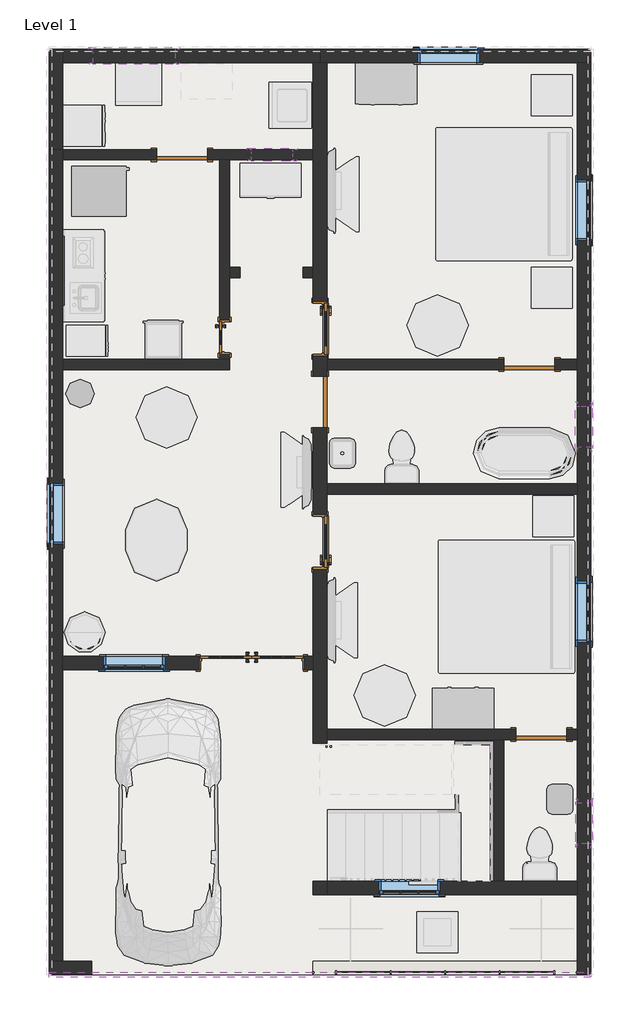
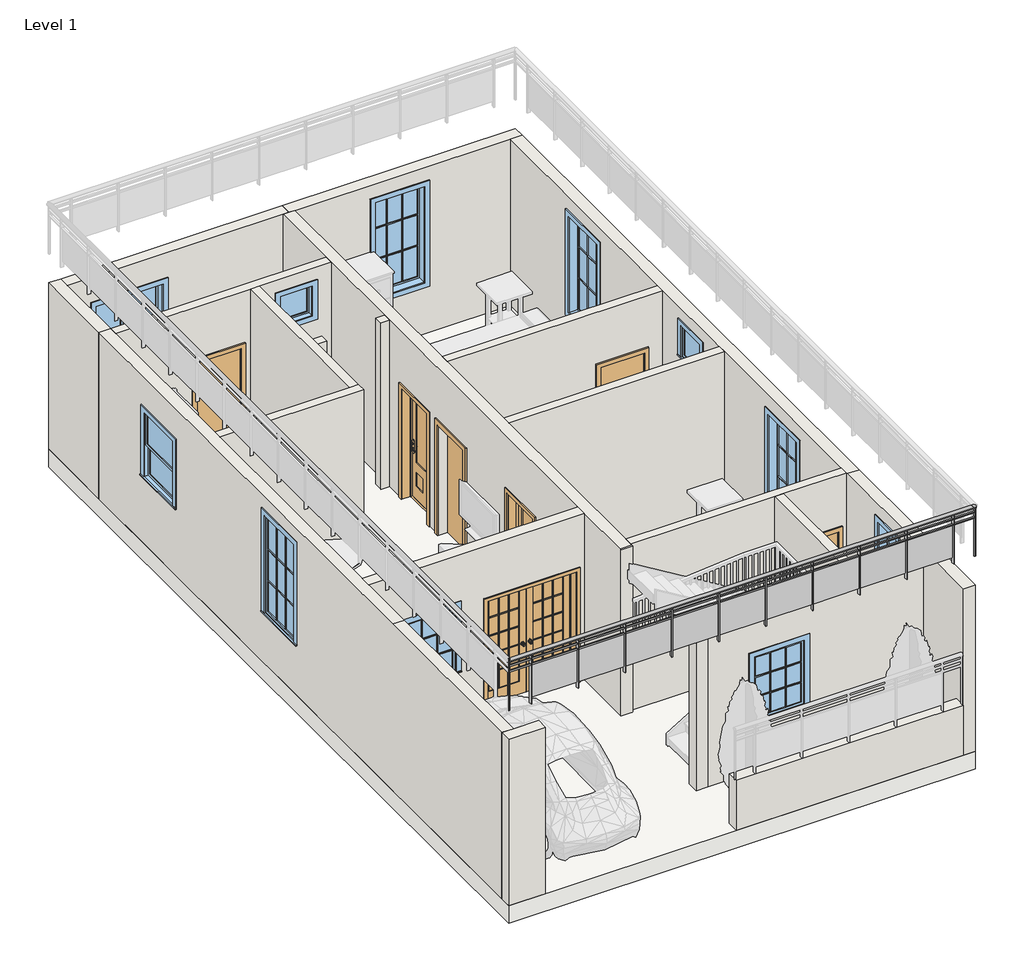
# One storey, part 1 of 3: 20 walls, 11 windows, 8 doors, 1 railing, 1 slab.
# Revit data of these elements (continued)
# Room at (-9273.472, 9026.088) mm, phase "New Construction", upper level "Level 1", upper offset 10' - 0", lower offset 0' - 0"
#   Number = "3"
#   Name = "Store"
# Room at (-6581.859, 9516.61) mm, phase "New Construction", upper level "Level 1", upper offset 10' - 0", lower offset 0' - 0"
#   Number = "4"
#   Name = "Master Bed"
# Room at (-6717.483, 6115.39) mm, phase "New Construction", upper level "Level 1", upper offset 10' - 0", lower offset 0' - 0"
#   Number = "5"
#   Name = "Toilet"
# Room at (-10587.98, 5145.157) mm, phase "New Construction", upper level "Level 1", upper offset 10' - 0", lower offset 0' - 0"
#   Number = "6"
# Room at (-6581.859, 3542.709) mm, phase "New Construction", upper level "Level 1", upper offset 10' - 0", lower offset 0' - 0"
#   Number = "7"
#   Name = "Bed Room"
# Room at (-5171.96, 0) mm, phase "New Construction", upper level "Level 1", upper offset 10' - 0", lower offset 0' - 0"
#   Number = "8"
#   Name = "Bath"
# Room at (-10587.98, -159.203) mm, phase "New Construction", upper level "Level 1", upper offset 10' - 0", lower offset 0' - 0"
#   Number = "9"
#   Name = "Porch"
